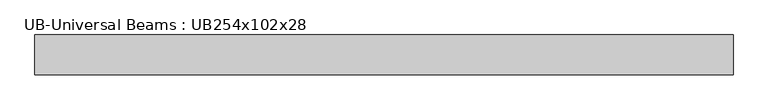
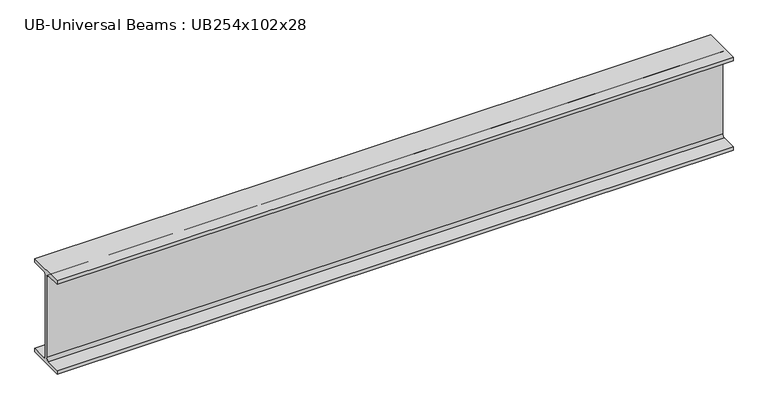
"""IFC4 building model written with IfcOpenShell, lengths in millimetres: beam geometry, UB-Universal Beams : UB254x102x28."""

from ifc_helpers import new_model, si_unit, point, frame, frame_2d, origin, place, context, project, spatial, polyline, circle_curve, trimmed, segment, composite_curve, outline, extrude, source, transform, mapped, element, save


def ub_universal_beams_ub254x102x28_93a23aa5(model_context):
    return source(origin(), model_context, "Body", "SweptSolid", [
        extrude(outline(composite_curve([segment(polyline([(51.1, -120.2), (51.1, -130.2), (-51.1, -130.2), (-51.1, -120.2), (-10.75, -120.2)]), True, "CONTINUOUS"), segment(trimmed(circle_curve(frame_2d((-10.75, -112.6)), 7.6), [point((-10.75, -120.2))], [point((-3.15, -112.6))], True, "CARTESIAN"), True, "CONTINUOUS"), segment(polyline([(-3.15, -112.6), (-3.15, 112.6)]), True, "CONTINUOUS"), segment(trimmed(circle_curve(frame_2d((-10.75, 112.6)), 7.6), [point((-3.15, 112.6))], [point((-10.75, 120.2))], True, "CARTESIAN"), True, "CONTINUOUS"), segment(polyline([(-10.75, 120.2), (-51.1, 120.2), (-51.1, 130.2), (51.1, 130.2), (51.1, 120.2), (10.75, 120.2)]), True, "CONTINUOUS"), segment(trimmed(circle_curve(frame_2d((10.75, 112.6)), 7.6), [point((10.75, 120.2))], [point((3.15, 112.6))], True, "CARTESIAN"), True, "CONTINUOUS"), segment(polyline([(3.15, 112.6), (3.15, -112.6)]), True, "CONTINUOUS"), segment(trimmed(circle_curve(frame_2d((10.75, -112.6)), 7.6), [point((3.15, -112.6))], [point((10.75, -120.2))], True, "CARTESIAN"), True, "CONTINUOUS"), segment(polyline([(10.75, -120.2), (51.1, -120.2)]), True, "CONTINUOUS")], self_intersect=False)), frame((-774.75, 0.0, 0.0), z_axis=(1.0, 0.0, 0.0), x_axis=(0.0, 1.0, 0.0)), (0.0, 0.0, 1.0), 1786.5),
    ])


if __name__ == "__main__":
    model = new_model("IFC4")
    model_context = context("Model", 3, world=origin())
    ifc_project = project(units=[si_unit("LENGTHUNIT", "METRE", prefix="MILLI")], contexts=[model_context])
    site = spatial("IfcSite", under=ifc_project)
    building = spatial("IfcBuilding", under=site)
    placement = place(None, origin())
    ub_universal_beams_ub254x102x28_shape = ub_universal_beams_ub254x102x28_93a23aa5(model_context)
    element("IfcBeam", 1, ObjectType="UB-Universal Beams : UB254x102x28", at=placement, inside=building, context=model_context, shape_type="MappedRepresentation", body=[
        mapped(ub_universal_beams_ub254x102x28_shape, transform((0.0, 0.0, 0.0), x_axis=(1.0, 0.0, 0.0), y_axis=(0.0, 1.0, 0.0), z_axis=(0.0, 0.0, 1.0))),
    ])
    save(model, "model.ifc")

# Revit data of these elements
# Type "UB-Universal Beams : UB254x102x28"
#   Section Name Key = "UB254X102X28"
#   Width = 10.22 cm
#   Web Thickness = 0.63 cm
#   Web Fillet = 0.76 cm
#   Warping Constant = 28000.0 cm⁶
#   Torsional Moment of Inertia = 9.57 cm⁴
#   Section Area = 36.1 cm²
#   Plastic Modulus weak axis = 54.8 cm³
#   Plastic Modulus strong axis = 353.0 cm³
#   Nominal Weight = 28.2999 kgf/m
#   Moment of Inertia weak axis = 179.00 cm⁴
#   Moment of Inertia strong axis = 4005.00 cm⁴
#   Height = 26.04 cm
#   Flange Thickness = 1.0 cm
#   Elastic Modulus weak axis = 34.9 cm³
#   Elastic Modulus strong axis = 308.0 cm³
#   Centroid Vertical = 13.02 cm
#   Centroid Horizontal = 5.11 cm
#   Bolt Spacing = 5.4 cm
#   Length [instance default] = 4' - 11.05512"
#   Structural Material [instance default] = Metal - Steel 43-275
#   Type Comments = ""
#   Assembly Code = ""
# Element 1 (IfcBeam, "UB-Universal Beams : UB254x102x28")
#   Materials on its faces: "Metal - Steel 43-275"
# Materials
#   "Metal - Steel 43-275": class "Metal", colour RGB 247 247 247, transparency 0, Cost = 0
